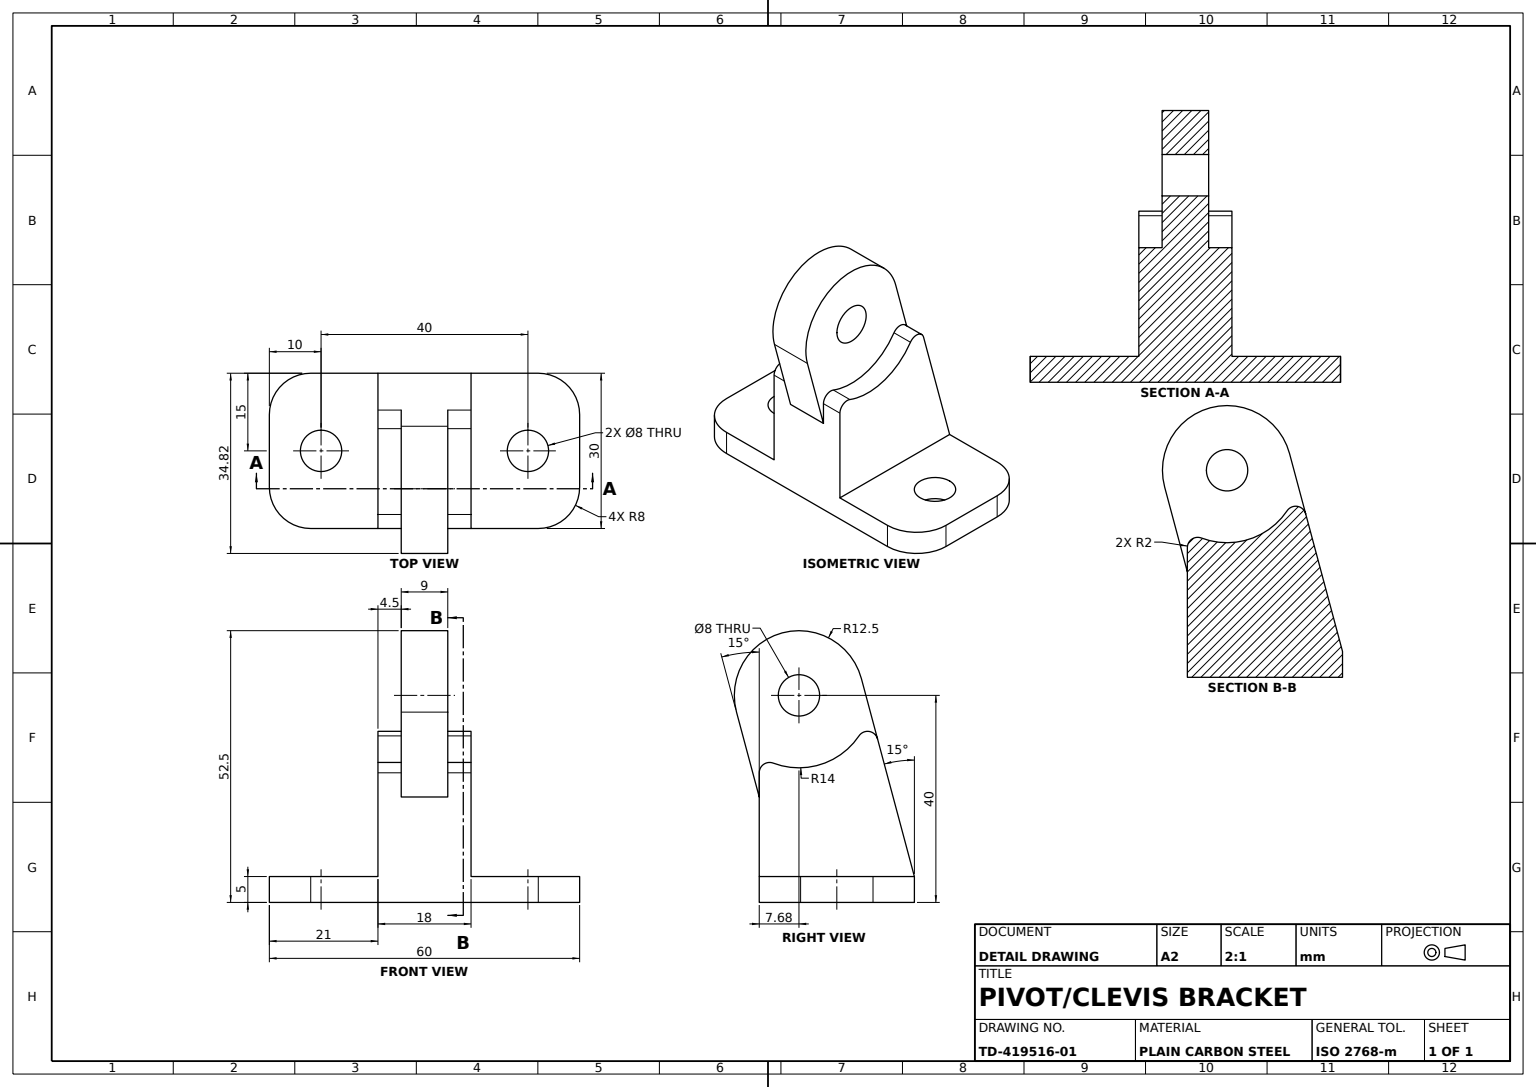
SolidWorks part; units mm, degrees
material "Plain Carbon Steel"
ref_plane "Front Plane" through (0, 0, 0) normal (0, 0, 1) x (1, 0, 0)
ref_plane "Top Plane" through (0, 0, 0) normal (0, 1, 0) x (1, 0, 0)
ref_plane "Right Plane" through (0, 0, 0) normal (1, 0, 0) x (0, 0, -1)
sketch "Base Plate Sketch" plane through (0, 0, 0) normal (0, 1, 0) x (1, 0, 0)
  line L0 (-20, 0) -> (20, 0) construction
  line L1 (-22, 15) -> (22, 15)
  line L2 (-30, 7) -> (-30, -7)
  line L3 (-22, -15) -> (22, -15)
  line L4 (30, 7) -> (30, -7)
  line L5 (-30, 15) -> (30, -15) construction
  line L6 (-30, -15) -> (30, 15) construction
  circle A0 centre (-20, 0) radius 4
  circle A1 centre (20, 0) radius 4
  arc A2 (-30, -7) -> (-22, -15) centre (-22, -7) ccw
  arc A3 (22, -15) -> (30, -7) centre (22, -7) ccw
  arc A4 (22, 15) -> (30, 7) centre (22, 7) cw
  arc A5 (-22, 15) -> (-30, 7) centre (-22, 7) ccw
  point P0 (0, 0)
  dimension "D4" = 8
  dimension "D5" = 8
  dimension "D1" = 60
  dimension "D2" = 30
  dimension "D3" = 40
extrude "Base Plate" add sketch "Base Plate Sketch" along normal blind 5
sketch "Tapered Upright Sketch" plane through (0, 0, 0) normal (1, 0, 0) x (0, 0, -1)
  line L0 (-15, 5) -> (-15, 20.3689)
  line L1 (15, 5) -> (4.7549, 43.2352)
  line L2 (-15, 5) -> (15, 5)
  line L3 (15, 5) -> (15, 0) construction
  line L4 (-19.3932, 36.7648) -> (-15, 20.3689)
  arc A0 (4.7549, 43.2352) -> (-19.3932, 36.7648) centre (-7.3192, 40) ccw
  circle A1 centre (-7.3192, 40) radius 4
  dimension "D3" = 25
  dimension "D4" = 8
  dimension "D1" = 40
  dimension "D2" = 15
extrude "Tapered Upright" add sketch "Tapered Upright Sketch" along normal mid plane 18
sketch "Pivot Lug Sketch" plane through (0, 0, 0) normal (1, 0, 0) x (0, 0, -1)
  line L0 (-15, 20.3689) -> (-15, 25.0425)
  line L4 (15, 5) -> (4.7549, 43.2352)
  line L5 (-19.3932, 36.7648) -> (-15, 20.3689)
  line L6 (-15, 20.3689) -> (-15, 5)
  line L7 (-15, 5) -> (15, 5)
  line L8 (7.8795, 31.5739) -> (4.7549, 43.2352)
  line L9 (-19.3932, 36.7648) -> (-15, 20.3689)
  arc A0 (-12.2899, 26.9121) -> (4.2893, 32.1742) centre (-7.3192, 40) ccw
  arc A1 (4.7549, 43.2352) -> (-19.3932, 36.7648) centre (-7.3192, 40) ccw
  arc A2 (4.7549, 43.2352) -> (-19.3932, 36.7648) centre (-7.3192, 40) ccw
  arc A3 (-12.2899, 26.9121) -> (-15, 25.0425) centre (-13, 25.0425) ccw
  arc A4 (7.8795, 31.5739) -> (4.2893, 32.1742) centre (5.9477, 31.0563) ccw
  dimension "D2" = 28
  dimension "D3" = 4
  dimension "D1" = 0
extrude "Pivot Lug" add sketch "Pivot Lug Sketch" along normal mid plane 20
sketch "Lug Side Relief Sketch" plane through (10, 0, 0) normal (1, 0, 0) x (0, 0, -1)
  line L3 (-19.3932, 36.7648) -> (-15, 20.3689)
  line L4 (-15, 20.3689) -> (-15, 25.0425)
  line L5 (7.8795, 31.5739) -> (4.7549, 43.2352)
  line L6 (-19.3932, 36.7648) -> (-15, 20.3689)
  line L7 (-15, 20.3689) -> (-15, 25.0425)
  line L8 (7.8795, 31.5739) -> (4.7549, 43.2352)
  arc A4 (4.7549, 43.2352) -> (-19.3932, 36.7648) centre (-7.3192, 40) ccw
  arc A5 (-12.2899, 26.9121) -> (-15, 25.0425) centre (-13, 25.0425) ccw
  arc A6 (-12.2899, 26.9121) -> (4.2893, 32.1742) centre (-7.3192, 40) ccw
  arc A7 (7.8795, 31.5739) -> (4.2893, 32.1742) centre (5.9477, 31.0563) ccw
  arc A8 (4.7549, 43.2352) -> (-19.3932, 36.7648) centre (-7.3192, 40) ccw
  arc A9 (-12.2899, 26.9121) -> (-15, 25.0425) centre (-13, 25.0425) ccw
  arc A10 (-12.2899, 26.9121) -> (4.2893, 32.1742) centre (-7.3192, 40) ccw
  arc A11 (7.8795, 31.5739) -> (4.2893, 32.1742) centre (5.9477, 31.0563) ccw
  dimension "D1" = 0
extrude "Lug Side Relief Cut" cut sketch "Lug Side Relief Sketch" against normal offset from surface (5.5 mm away) 4.5 up to plane "Right Plane"
mirror "Lug Side Relief Mirror" about plane through (0, 0, 0) normal (1, 0, 0) of "Lug Side Relief Cut"
sketch "Pivot Bore Sketch" plane through (4.5, 0, 0) normal (1, 0, 0) x (0, 0, -1)
  circle A0 centre (-7.3192, 40) radius 4
  dimension "D1" = 8
extrude "Pivot Bore Ø8" cut sketch "Pivot Bore Sketch" against normal through all
